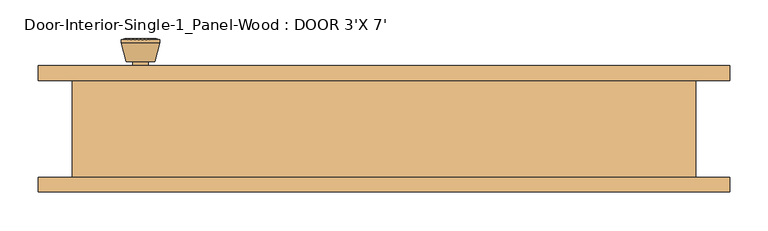
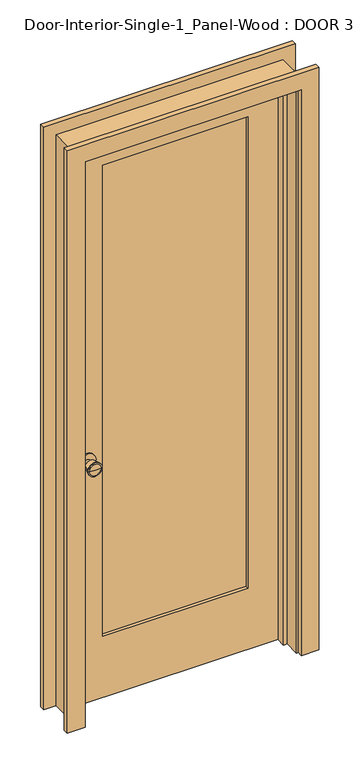
"""IFC4 building model written with IfcOpenShell, lengths in millimetres: door geometry, Door-Interior-Single-1_Panel-Wood : DOOR 3'X 7'."""

from ifc_helpers import new_model, si_unit, point, frame, frame_2d, origin, place, context, project, spatial, polyline, circle_curve, trimmed, segment, composite_curve, outline, extrude, faceted_brep, source, transform, mapped, element, save
from ifc_brep_helpers import plane_surface, cylinder_surface, revolved_surface, advanced_brep


def door_interior_single_1_panel_wood_door_3_x_7_d4f3ff50(model_context):
    return source(origin(), model_context, "Body", "SolidModel", [
        advanced_brep(
        [(-317.5, 19.4, 914.4), (-307.5, 19.4, 914.4), (-327.5, 19.4, 914.4), (-297.0241324, -29.6, 914.4), (-317.5, -29.6, 914.4), (-337.9758676, -29.6, 914.4), (-292.5, -27.7721319, 914.4), (-342.5, -27.7721319, 914.4), (-292.5, -24.3084537, 914.4), (-342.5, -24.3084537, 914.4), (-298.863764, 0.4, 914.4), (-336.136236, 0.4, 914.4), (-307.5, 0.4, 914.4), (-327.5, 0.4, 914.4)],
        [
            (0, 1),
            (1, 2, circle_curve(frame((-317.5, 19.4, 914.4), z_axis=(0.0, 1.0, 0.0), x_axis=(-1.0, 0.0, 0.0)), 10.0)),
            (2, 0),
            (2, 1, circle_curve(frame((-317.5, 19.4, 914.4), z_axis=(0.0, 1.0, 0.0), x_axis=(-1.0, 0.0, 0.0)), 10.0)),
            (3, 4),
            (4, 5),
            (5, 3, circle_curve(frame((-317.5, -29.6, 914.4), z_axis=(0.0, -1.0, 0.0), x_axis=(-1.0, 0.0, 0.0)), 20.4758676)),
            (3, 5, circle_curve(frame((-317.5, -29.6, 914.4), z_axis=(0.0, -1.0, 0.0), x_axis=(-1.0, 0.0, 0.0)), 20.4758676)),
            (6, 3),
            (5, 7),
            (7, 6, circle_curve(frame((-317.5, -27.7721319, 914.4), z_axis=(0.0, -1.0, 0.0), x_axis=(-1.0, 0.0, 0.0)), 25.0)),
            (6, 7, circle_curve(frame((-317.5, -27.7721319, 914.4), z_axis=(0.0, -1.0, 0.0), x_axis=(-1.0, 0.0, 0.0)), 25.0)),
            (8, 6),
            (7, 9),
            (9, 8, circle_curve(frame((-317.5, -24.3084537, 914.4), z_axis=(0.0, -1.0, 0.0), x_axis=(-1.0, 0.0, 0.0)), 25.0)),
            (8, 9, circle_curve(frame((-317.5, -24.3084537, 914.4), z_axis=(0.0, -1.0, 0.0), x_axis=(-1.0, 0.0, 0.0)), 25.0)),
            (10, 8),
            (9, 11),
            (11, 10, circle_curve(frame((-317.5, 0.4, 914.4), z_axis=(0.0, -1.0, 0.0), x_axis=(-1.0, 0.0, 0.0)), 18.636236)),
            (10, 11, circle_curve(frame((-317.5, 0.4, 914.4), z_axis=(0.0, -1.0, 0.0), x_axis=(-1.0, 0.0, 0.0)), 18.636236)),
            (12, 10),
            (11, 13),
            (13, 12, circle_curve(frame((-317.5, 0.4, 914.4), z_axis=(0.0, -1.0, 0.0), x_axis=(-1.0, 0.0, 0.0)), 10.0)),
            (12, 13, circle_curve(frame((-317.5, 0.4, 914.4), z_axis=(0.0, -1.0, 0.0), x_axis=(-1.0, 0.0, 0.0)), 10.0)),
            (1, 12),
            (13, 2),
        ],
        [
            plane_surface(frame((-317.5, 19.4, 914.4), z_axis=(0.0, 1.0, 0.0), x_axis=(-1.0, 0.0, 0.0))),
            plane_surface(frame((-317.5, -29.6, 914.4), z_axis=(0.0, -1.0, 0.0), x_axis=(-1.0, 0.0, 0.0))),
            revolved_surface(polyline([(-337.9758676, -29.6, 914.4), (-342.5, -27.7721319, 914.4)]), (-317.5, 19.4, 914.4), (0.0, 1.0, 0.0)),
            cylinder_surface(frame((-317.5, 19.4, 914.4), z_axis=(0.0, 1.0, 0.0), x_axis=(-1.0, 0.0, 0.0)), 25.0),
            revolved_surface(polyline([(-342.5, -24.3084537, 914.4), (-336.136236, 0.4, 914.4)]), (-317.5, 19.4, 914.4), (0.0, 1.0, 0.0)),
            plane_surface(frame((-317.5, 0.4, 914.4), z_axis=(0.0, 1.0, 0.0), x_axis=(-1.0, 0.0, 0.0))),
            cylinder_surface(frame((-317.5, 19.4, 914.4), z_axis=(0.0, 1.0, 0.0), x_axis=(-1.0, 0.0, 0.0)), 10.0),
        ],
        [
            (0, [[1, 2, 3]]),
            (0, [[-3, 4, -1]]),
            (1, [[5, 6, 7]]),
            (1, [[-6, -5, 8]]),
            (2, [[9, -7, 10, 11]]),
            (2, [[-10, -8, -9, 12]]),
            (3, [[13, -11, 14, 15]]),
            (3, [[-14, -12, -13, 16]]),
            (4, [[17, -15, 18, 19]]),
            (4, [[-18, -16, -17, 20]]),
            (5, [[21, -19, 22, 23]]),
            (5, [[-22, -20, -21, 24]]),
            (6, [[25, -23, 26, -2]]),
            (6, [[-26, -24, -25, -4]]),
        ],
    ),
        extrude(outline(composite_curve([segment(trimmed(circle_curve(frame_2d((914.4, -317.5)), 30.0), [point((914.4, -347.5))], [point((914.4, -287.5))], False, "CARTESIAN"), True, "CONTINUOUS"), segment(trimmed(circle_curve(frame_2d((914.4, -317.5)), 30.0), [point((914.4, -287.5))], [point((914.4, -347.5))], False, "CARTESIAN"), True, "CONTINUOUS")], self_intersect=False)), frame((0.0, 19.4, 0.0), z_axis=(0.0, 1.0, 0.0), x_axis=(0.0, 0.0, 1.0)), (0.0, 0.0, 1.0), 6.0),
        advanced_brep(
        [(-317.5, 66.325, 914.4), (-327.5, 66.325, 914.4), (-307.5, 66.325, 914.4), (-297.0241324, 115.325, 914.4), (-337.9758676, 115.325, 914.4), (-317.5, 115.325, 914.4), (-292.5, 113.4971319, 914.4), (-342.5, 113.4971319, 914.4), (-292.5, 110.0334537, 914.4), (-342.5, 110.0334537, 914.4), (-298.863764, 85.325, 914.4), (-336.136236, 85.325, 914.4), (-307.5, 85.325, 914.4), (-327.5, 85.325, 914.4)],
        [
            (0, 1),
            (1, 2, circle_curve(frame((-317.5, 66.325, 914.4), z_axis=(0.0, -1.0, 0.0), x_axis=(-1.0, 0.0, 0.0)), 10.0)),
            (2, 0),
            (2, 1, circle_curve(frame((-317.5, 66.325, 914.4), z_axis=(0.0, -1.0, 0.0), x_axis=(-1.0, 0.0, 0.0)), 10.0)),
            (3, 4, circle_curve(frame((-317.5, 115.325, 914.4), z_axis=(0.0, 1.0, 0.0), x_axis=(-1.0, 0.0, 0.0)), 20.4758676)),
            (4, 5),
            (5, 3),
            (4, 3, circle_curve(frame((-317.5, 115.325, 914.4), z_axis=(0.0, 1.0, 0.0), x_axis=(-1.0, 0.0, 0.0)), 20.4758676)),
            (6, 7, circle_curve(frame((-317.5, 113.4971319, 914.4), z_axis=(0.0, 1.0, 0.0), x_axis=(-1.0, 0.0, 0.0)), 25.0)),
            (7, 4),
            (3, 6),
            (7, 6, circle_curve(frame((-317.5, 113.4971319, 914.4), z_axis=(0.0, 1.0, 0.0), x_axis=(-1.0, 0.0, 0.0)), 25.0)),
            (8, 9, circle_curve(frame((-317.5, 110.0334537, 914.4), z_axis=(0.0, 1.0, 0.0), x_axis=(-1.0, 0.0, 0.0)), 25.0)),
            (9, 7),
            (6, 8),
            (9, 8, circle_curve(frame((-317.5, 110.0334537, 914.4), z_axis=(0.0, 1.0, 0.0), x_axis=(-1.0, 0.0, 0.0)), 25.0)),
            (10, 11, circle_curve(frame((-317.5, 85.325, 914.4), z_axis=(0.0, 1.0, 0.0), x_axis=(-1.0, 0.0, 0.0)), 18.636236)),
            (11, 9),
            (8, 10),
            (11, 10, circle_curve(frame((-317.5, 85.325, 914.4), z_axis=(0.0, 1.0, 0.0), x_axis=(-1.0, 0.0, 0.0)), 18.636236)),
            (12, 13, circle_curve(frame((-317.5, 85.325, 914.4), z_axis=(0.0, 1.0, 0.0), x_axis=(-1.0, 0.0, 0.0)), 10.0)),
            (13, 11),
            (10, 12),
            (13, 12, circle_curve(frame((-317.5, 85.325, 914.4), z_axis=(0.0, 1.0, 0.0), x_axis=(-1.0, 0.0, 0.0)), 10.0)),
            (1, 13),
            (12, 2),
        ],
        [
            plane_surface(frame((-317.5, 66.325, 914.4), z_axis=(0.0, -1.0, 0.0), x_axis=(-1.0, 0.0, 0.0))),
            plane_surface(frame((-317.5, 115.325, 914.4), z_axis=(0.0, 1.0, 0.0), x_axis=(-1.0, 0.0, 0.0))),
            revolved_surface(polyline([(-337.9758676, 115.325, 914.4), (-342.5, 113.4971319, 914.4)]), (-317.5, 66.325, 914.4), (0.0, -1.0, 0.0)),
            cylinder_surface(frame((-317.5, 66.325, 914.4), z_axis=(0.0, -1.0, 0.0), x_axis=(-1.0, 0.0, 0.0)), 25.0),
            revolved_surface(polyline([(-342.5, 110.0334537, 914.4), (-336.136236, 85.325, 914.4)]), (-317.5, 66.325, 914.4), (0.0, -1.0, 0.0)),
            plane_surface(frame((-317.5, 85.325, 914.4), z_axis=(0.0, -1.0, 0.0), x_axis=(-1.0, 0.0, 0.0))),
            cylinder_surface(frame((-317.5, 66.325, 914.4), z_axis=(0.0, -1.0, 0.0), x_axis=(-1.0, 0.0, 0.0)), 10.0),
        ],
        [
            (0, [[1, 2, 3]]),
            (0, [[-3, 4, -1]]),
            (1, [[5, 6, 7]]),
            (1, [[8, -7, -6]]),
            (2, [[9, 10, -5, 11]]),
            (2, [[12, -11, -8, -10]]),
            (3, [[13, 14, -9, 15]]),
            (3, [[16, -15, -12, -14]]),
            (4, [[17, 18, -13, 19]]),
            (4, [[20, -19, -16, -18]]),
            (5, [[21, 22, -17, 23]]),
            (5, [[24, -23, -20, -22]]),
            (6, [[-2, 25, -21, 26]]),
            (6, [[-4, -26, -24, -25]]),
        ],
    ),
        extrude(outline(composite_curve([segment(trimmed(circle_curve(frame_2d((914.4, -317.5)), 30.0), [point((914.4, -347.5))], [point((914.4, -287.5))], False, "CARTESIAN"), True, "CONTINUOUS"), segment(trimmed(circle_curve(frame_2d((914.4, -317.5)), 30.0), [point((914.4, -287.5))], [point((914.4, -347.5))], False, "CARTESIAN"), True, "CONTINUOUS")], self_intersect=False)), frame((0.0, 60.325, 0.0), z_axis=(0.0, 1.0, 0.0), x_axis=(0.0, 0.0, 1.0)), (0.0, 0.0, 1.0), 6.0),
        faceted_brep([(406.4, 60.325, 0.0), (406.4, -66.675, 0.0), (381.0, -66.675, 0.0), (381.0, -9.525, 0.0), (368.3, -9.525, 0.0), (368.3, 25.4, 0.0), (381.0, 25.4, 0.0), (381.0, 60.325, 0.0), (406.4, 60.325, 2159.0), (406.4, -66.675, 2159.0), (-406.4, -66.675, 2159.0), (-406.4, -66.675, 0.0), (-381.0, -66.675, 0.0), (-381.0, -66.675, 2133.6), (381.0, -66.675, 2133.6), (381.0, -9.525, 2133.6), (-381.0, -9.525, 2133.6), (-381.0, -9.525, 0.0), (-368.3, -9.525, 0.0), (-368.3, -9.525, 2120.9), (368.3, -9.525, 2120.9), (368.3, 25.4, 2120.9), (-368.3, 25.4, 2120.9), (-368.3, 25.4, 0.0), (-381.0, 25.4, 0.0), (-381.0, 25.4, 2133.6), (381.0, 25.4, 2133.6), (381.0, 60.325, 2133.6), (-381.0, 60.325, 2133.6), (-381.0, 60.325, 0.0), (-406.4, 60.325, 0.0), (-406.4, 60.325, 2159.0)], [[[0, 1, 2, 3, 4, 5, 6, 7]], [[1, 0, 8, 9]], [[2, 1, 9, 10, 11, 12, 13, 14]], [[3, 2, 14, 15]], [[4, 3, 15, 16, 17, 18, 19, 20]], [[5, 4, 20, 21]], [[6, 5, 21, 22, 23, 24, 25, 26]], [[7, 6, 26, 27]], [[0, 7, 27, 28, 29, 30, 31, 8]], [[9, 8, 31, 10]], [[15, 14, 13, 16]], [[21, 20, 19, 22]], [[27, 26, 25, 28]], [[30, 29, 24, 23, 18, 17, 12, 11]], [[10, 31, 30, 11]], [[16, 13, 12, 17]], [[22, 19, 18, 23]], [[28, 25, 24, 29]]]),
        extrude(outline(polyline([(2133.6, -381.0), (0.0, -381.0), (0.0, 381.0), (2133.6, 381.0), (2133.6, -381.0)]), holes=[polyline([(2014.5375, -260.35), (2014.5375, 260.35), (231.775, 260.35), (231.775, -260.35), (2014.5375, -260.35)])]), frame((0.0, 25.4, 0.0), z_axis=(0.0, 1.0, 0.0), x_axis=(0.0, 0.0, 1.0)), (0.0, 0.0, 1.0), 34.925),
        extrude(outline(polyline([(260.35, 37.0416667), (-260.35, 37.0416667), (-260.35, 48.6833333), (260.35, 48.6833333), (260.35, 37.0416667)])), frame((0.0, 0.0, 231.775), z_axis=(0.0, 0.0, 1.0), x_axis=(1.0, 0.0, 0.0)), (0.0, 0.0, 1.0), 1782.7625),
        extrude(outline(polyline([(0.0, 387.35), (0.0, 450.85), (2203.45, 450.85), (2203.45, -450.85), (0.0, -450.85), (0.0, -387.35), (2139.95, -387.35), (2139.95, 387.35), (0.0, 387.35)])), frame((0.0, 60.325, 0.0), z_axis=(0.0, 1.0, 0.0), x_axis=(0.0, 0.0, 1.0)), (0.0, 0.0, 1.0), 19.05),
        extrude(outline(polyline([(0.0, 387.35), (0.0, 450.85), (2203.45, 450.85), (2203.45, -450.85), (0.0, -450.85), (0.0, -387.35), (2139.95, -387.35), (2139.95, 387.35), (0.0, 387.35)])), frame((0.0, -85.725, 0.0), z_axis=(0.0, 1.0, 0.0), x_axis=(0.0, 0.0, 1.0)), (0.0, 0.0, 1.0), 19.05),
    ])


if __name__ == "__main__":
    model = new_model("IFC4")
    model_context = context("Model", 3, world=origin())
    ifc_project = project(units=[si_unit("LENGTHUNIT", "METRE", prefix="MILLI")], contexts=[model_context])
    site = spatial("IfcSite", under=ifc_project)
    building = spatial("IfcBuilding", under=site)
    placement = place(None, origin())
    door_interior_single_1_panel_wood_door_3_x_7_shape = door_interior_single_1_panel_wood_door_3_x_7_d4f3ff50(model_context)
    element("IfcDoor", 1, ObjectType="Door-Interior-Single-1_Panel-Wood : DOOR 3'X 7'", at=placement, inside=building, context=model_context, shape_type="MappedRepresentation", body=[
        mapped(door_interior_single_1_panel_wood_door_3_x_7_shape, transform((0.0, 0.0, 0.0), x_axis=(1.0, 0.0, 0.0), y_axis=(0.0, 1.0, 0.0), z_axis=(0.0, 0.0, 1.0))),
    ])
    save(model, "model.ifc")

# Revit data of these elements
# Type "Door-Interior-Single-1_Panel-Wood : DOOR 3'X 7'"
#   Type Mark = "11"
#   Assembly Code = "C1020300"
#   Analytic Construction = "Wooden"
#   Top Rail = 0' - 4 11/16"
#   Thickness = 0' - 1 3/8"
#   Thermal Resistance (R) = 2.5876 (h·ft²·°F)/BTU
#   Swing Angle [instance default] = 90.00°
#   Stiles = 0' - 4 3/4"
#   Rough Width = 2' - 8"
#   Rough Height = 7' - 1"
#   Height = 7' - 0"
#   Width = 2' - 6"
#   Heat Transfer Coefficient (U) = 0.3865 BTU/(h·ft²·°F)
#   Bottom Rail = 0' - 9 1/8"
#   Trim Material = Cherry
#   Panel Material = Cherry
#   Frame Material = Cherry
#   Door Handle Material = Aluminum
#   Visual Light Transmittance = 0
#   Solar Heat Gain Coefficient = 0
#   Wall Closure = (empty or 0)
#   Function = (empty or 0)
# Element 1 (IfcDoor, "Door-Interior-Single-1_Panel-Wood : DOOR 3'X 7'")
#   Materials on its faces: "Cherry", "Aluminum"
# Materials
#   "Cherry": class "Wood", colour RGB 226 177 128, transparency 0, Description = "Prunus Serotina", Cost = 0
#   "Aluminum": class "Metal", colour RGB 247 247 247, transparency 0, Description = "Aluminum 6061", Cost = 0
